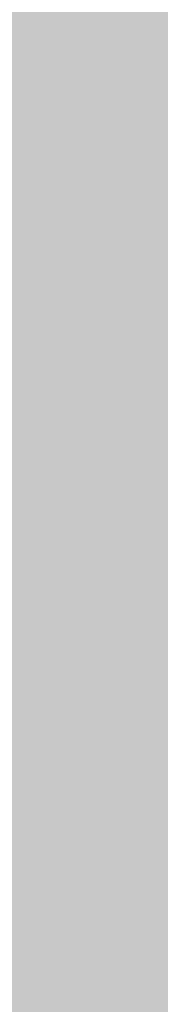
# Model space of a CAD drawing. Units: inches. Extents: x 2083 to 3317, y 1141 to 2115.
# Tile 168 of 256: x 3126.958245 to 3126.959398, y 1263.265937 to 1263.274018. Entities that reach past the tile are written whole.
import ezdxf

# ---------------------------------------------------------------- set-up
doc = ezdxf.new("R2010")
doc.units = ezdxf.units.IN
doc.layers.add('A-ANNO-DIMS', color=2, linetype='Continuous', lineweight=18)
doc.layers.add('A-WALL-PATT', color=251, linetype='Continuous', lineweight=13, true_color=0x636466)
doc.styles.get("Standard").update_dxf_attribs({"font": 'arial.ttf'})
doc.dimstyles.new('ISO-25', dxfattribs={"dimtxt": 12, "dimasz": 12, "dimexe": 1.25, "dimexo": 0.625, "dimtad": 1, "dimlunit": 3, "dimtxsty": 'Standard', "dimcen": 2.5, "dimadec": 0, "dimazin": 0, "dimtfac": 1, "dimtmove": 0, "dimatfit": 3, "dimfxl": 1, "dimarcsym": 0})

# ---------------------------------------------------------------- blocks, each defined once
blk = doc.blocks.new('*D26')
at = {"layer": 'A-ANNO-DIMS', "color": 0, "lineweight": -2, "transparency": 16777216}
for p, q in [((3088.985844, 1274.915092), (3088.985844, 1270.9519631)), ((3111.2400366, 1274.915092), (3111.2400366, 1270.9519631)), ((3076.985844, 1272.2019631), (2840.262447, 1272.2019631)), ((3111.2400366, 1272.2019631), (3088.985844, 1272.2019631)), ((3123.2400366, 1272.2019631), (3135.2400366, 1272.2019631))]:
    blk.add_line(p, q, dxfattribs=at)
at = {"layer": 'A-ANNO-DIMS', "color": 0, "transparency": 16777216}
for points in [[(3076.985844, 1274.2019631), (3076.985844, 1270.2019631), (3088.985844, 1272.2019631)], [(3123.2400366, 1274.2019631), (3123.2400366, 1270.2019631), (3111.2400366, 1272.2019631)]]:
    blk.add_solid(points, dxfattribs=at)
at = {"layer": 'Defpoints', "color": 0, "transparency": 16777216}
for p in [(3088.985844, 1275.540092), (3111.2400366, 1275.540092), (3088.985844, 1272.2019631)]:
    blk.add_point(p, dxfattribs=at)
at = {"layer": 'A-ANNO-DIMS', "color": 0, "transparency": 16777216, "insert": (2952.6241455, 1279.0316016), "char_height": 12, "attachment_point": 5}
blk.add_mtext('NIGHTSTAND 1\'-10 1/2" TYP.', dxfattribs=at)

msp = doc.modelspace()

# ---------------------------------------------------------------- hatches: boundary and pattern name
at = {"layer": 'A-WALL-PATT'}
h = msp.add_hatch(color=256, dxfattribs=at)
h.dxf.hatch_style = 1
h.paths.add_polyline_path([(3126.9597832, 2020.7613601), (2748.9597832, 2020.7613601), (2604.9597832, 2020.7613601), (2226.9597832, 2020.7613601), (2226.9597832, 1702.7613601), (2466.9597832, 1702.7613601), (2466.9597832, 1582.7613601), (2418.9597832, 1582.7613601), (2418.9597832, 1477.7613601), (2226.9597832, 1477.7613601), (2226.9597832, 1263.2613601), (2544.9597832, 1263.2613601), (2544.9597832, 1411.7613601), (2604.9597832, 1411.7613601), (2685.9597832, 1411.7613601), (2685.9597832, 1420.7613601), (2604.9597832, 1420.7613601), (2604.9597832, 1573.7613601), (2604.9597832, 1702.7613601), (2604.9597832, 2011.7613601), (2748.9597832, 2011.7613601), (2748.9597832, 1702.7613601), (2862.9597832, 1702.7613601), (2862.9597832, 1621.7613601), (2871.9597832, 1621.7613601), (2871.9597832, 1702.7613601), (2883.9597832, 1702.7613601), (2883.9597832, 1706.9394595, -0.026459), (2883.9597832, 1711.7613601), (2757.9597832, 1711.7613601), (2757.9597832, 1807.7613601), (2787.9597832, 1807.7613601), (2787.9597832, 1812.2613601), (2757.9597832, 1812.2613601), (2757.9597832, 2011.7613601), (2877.9597832, 2011.7613601), (2877.9597832, 1812.2613601), (2847.9597832, 1812.2613601), (2847.9597832, 1807.7613601), (2889.8357425, 1807.7613601), (2889.8357425, 1812.2613601), (2882.4597832, 1812.2613601), (2882.4597832, 2011.7613601), (3117.9597832, 2011.7613601), (3117.9597832, 1812.2613601), (2937.8357425, 1812.2613601), (2937.8357425, 1807.7613601), (2995.7097832, 1807.7613601), (2995.7097832, 1796.1176655), (3000.2097832, 1796.1176655), (3000.2097832, 1807.7613601), (3117.9597832, 1807.7613601), (3117.9597832, 1711.7613601), (3000.2097832, 1711.7613601), (3000.2097832, 1760.1176655), (2998.5727047, 1760.1176655, -0.020711), (2995.7097832, 1760.1176655), (2995.7097832, 1711.7613601), (2931.9597832, 1711.7613601), (2931.9597832, 1702.7613601), (3126.9597832, 1702.7613601)])
h.paths.add_polyline_path([(2471.4597832, 2011.7613601), (2471.4597832, 1810.0113601), (2462.7169357, 1810.0113601), (2462.7169357, 1805.5113601), (2505.9597832, 1805.5113601), (2505.9597832, 1810.0113601), (2475.9597832, 1810.0113601), (2475.9597832, 2011.7613601), (2595.9597832, 2011.7613601), (2595.9597832, 1810.0113601), (2565.9597832, 1810.0113601), (2565.9597832, 1805.5113601), (2595.9597832, 1805.5113601), (2595.9597832, 1711.7613601), (2235.9597832, 1711.7613601), (2235.9597832, 1805.5113601), (2353.7097832, 1805.5113601), (2353.7097832, 1796.0541624), (2358.2097832, 1796.0541624), (2358.2097832, 1805.5113601), (2414.7169357, 1805.5113601), (2414.7169357, 1810.0113601), (2235.9597832, 1810.0113601), (2235.9597832, 2011.7613601)], flags=16)
h.paths.add_polyline_path([(2270.2047343, 1994.6100082), (2270.2047343, 1970.6100082), (2246.2047343, 1970.6100082), (2246.2047343, 1994.6100082)], flags=0)
edge = h.paths.add_edge_path(flags=0)
edge.add_ellipse((2332.027391, 1899.7981761), major_axis=(-3.0429938, 3.0429938), ratio=0.16825245, start_angle=-161.3321656, end_angle=-156.3071136, ccw=False)
edge.add_ellipse((2333.0820373, 1898.7435297), major_axis=(-1.0546463, 1.0546463), ratio=0.453532097, start_angle=-123.371019, end_angle=-94.1591066)
edge = h.paths.add_edge_path(flags=0)
edge.add_ellipse((2332.027391, 1968.8762897), major_axis=(3.0429938, 3.0429938), ratio=0.16825245, start_angle=18.6678344, end_angle=23.6928864)
edge.add_spline(control_points=[(2332.9255964, 1970.6911045), (2332.2267681, 1970.3360997), (2330.8937087, 1969.6589054), (2328.4130803, 1970.9321376), (2327.2039345, 1967.7487119), (2324.7095965, 1969.9555886), (2322.5328223, 1967.012354), (2320.0128462, 1971.2958124), (2317.6803077, 1968.1578449), (2316.0405263, 1967.1020468), (2315.4269045, 1966.8096022)], knot_values=[0, 0, 0, 0, 2.267059, 4.324559, 6.685584, 8.878641, 11.121502, 14.300359, 17.755284, 19.732645, 19.732645, 19.732645, 19.732645], degree=3, periodic=0)
edge.add_ellipse((2332.027391, 1968.8762897), major_axis=(3.0429938, 3.0429938), ratio=0.16825245, start_angle=18.6678344, end_angle=23.6928864, ccw=False)
edge.add_ellipse((2333.0820373, 1969.930936), major_axis=(1.0546463, 1.0546463), ratio=0.453532097, start_angle=56.628981, end_angle=85.8408934, ccw=False)
edge = h.paths.add_edge_path(flags=0)
edge.add_spline(control_points=[(2296.4282874, 1967.9879081), (2293.6278045, 1965.3363137), (2287.7036238, 1959.727094), (2299.7438601, 1949.9956993), (2294.5325909, 1935.6685275), (2290.5732281, 1920.6035119), (2293.3941244, 1909.9736911), (2296.1854073, 1904.9665431)], knot_values=[0.099185, 0.099185, 0.099185, 0.099185, 0.345301, 0.619822, 0.982653, 1.386093, 1.810555, 1.810555, 1.810555, 1.810555], degree=3, periodic=0)
edge.add_spline(control_points=[(2296.1854073, 1904.9665431), (2297.3835817, 1902.6193002), (2298.0009694, 1901.9493116), (2298.5529698, 1901.4681549)], knot_values=[0.006246, 0.006246, 0.006246, 0.006246, 0.055476, 0.055476, 0.055476, 0.055476], degree=3, periodic=0)
edge.add_spline(control_points=[(2298.5529698, 1901.4681549), (2297.2586121, 1900.9232238), (2295.2252939, 1900.2321257), (2293.0602287, 1900.6142053), (2292.1014227, 1900.788415), (2292.0895776, 1900.790568)], knot_values=[0.312835, 0.312835, 0.312835, 0.312835, 0.40178, 0.474987, 0.475903, 0.475903, 0.475903, 0.475903], degree=3, periodic=0)
edge.add_arc((2292.7936464, 1904.6641088), 3.9370079, 215.4208969, 259.6981795, ccw=False)
edge.add_spline(control_points=[(2289.5853139, 1902.3823039), (2289.4766524, 1902.5350874), (2289.3684805, 1902.6880353), (2289.2608648, 1902.8411699)], knot_values=[0.102872, 0.102872, 0.102872, 0.102872, 0.116896, 0.116896, 0.116896, 0.116896], degree=3, periodic=0)
edge.add_spline(control_points=[(2289.2608648, 1902.8411699), (2288.6866042, 1902.5501922), (2287.6400477, 1902.0199025), (2285.8813368, 1901.8739536), (2283.8529717, 1901.5043521), (2281.7199871, 1899.7105375), (2278.4669913, 1899.492942), (2276.1571361, 1901.8832022), (2272.2589526, 1899.8040711), (2267.7776054, 1901.8431828), (2262.2438819, 1900.1840326), (2257.414927, 1901.7820606), (2254.318374, 1900.7261196), (2253.1782849, 1900.3373431)], knot_values=[0, 0, 0, 0, 1.907977, 3.477176, 5.261074, 7.972851, 11.680248, 13.717921, 16.939592, 22.789562, 27.502503, 33.595215, 37.145618, 37.145618, 37.145618, 37.145618], degree=3, periodic=0)
edge.add_line((2253.1782849, 1900.3373431), (2250.2442397, 1902.8411699))
edge.add_line((2250.2442397, 1902.8411699), (2250.2442397, 1965.8332959))
edge.add_line((2250.2442397, 1965.8332959), (2253.1782849, 1968.3371226))
edge.add_spline(control_points=[(2253.1782849, 1968.3371226), (2254.318374, 1967.9483462), (2257.414927, 1966.8924051), (2262.2438819, 1968.4904332), (2267.7776054, 1966.8312829), (2271.5267301, 1968.5372172), (2273.8759143, 1967.8282895), (2274.2067012, 1967.7276424)], knot_values=[0, 0, 0, 0, 0.09018, 0.244935, 0.364644, 0.513233, 0.537855, 0.537855, 0.537855, 0.537855], degree=3, periodic=0)
edge.add_arc((2274.3528869, 1963.7933495), 3.9370079, 72.0511336, 92.1279492, ccw=False)
edge.add_arc((2281.2969331, 1985.2300027), 18.5962982, 252.05113361, 288.56572166)
edge.add_arc((2292.3167172, 1956.0288805), 12.6460805, 71.02678788, 113.77821843, ccw=False)
edge = h.paths.add_edge_path(flags=0)
edge.add_spline(control_points=[(2274.8994147, 1951.8561946), (2275.066156, 1951.6165924), (2275.2326866, 1951.3765878), (2275.3979871, 1951.1358545)], knot_values=[1.409916, 1.409916, 1.409916, 1.409916, 1.43159, 1.43159, 1.43159, 1.43159], degree=3, periodic=0)
edge.add_spline(control_points=[(2275.3979871, 1951.1358545), (2275.7921055, 1950.5618854), (2276.1792311, 1949.9837745), (2276.5455462, 1949.3971029)], knot_values=[1.358238, 1.358238, 1.358238, 1.358238, 1.409916, 1.409916, 1.409916, 1.409916], degree=3, periodic=0)
edge.add_line((2276.5455462, 1949.3971029), (2277.437289, 1947.8621847))
edge.add_spline(control_points=[(2277.437289, 1947.8621847), (2276.3038341, 1945.6731147), (2274.6396979, 1942.4268817), (2274.631615, 1938.0938998), (2272.7991237, 1930.8515498), (2274.3564261, 1943.8970461), (2275.9476814, 1947.9233558), (2276.5455462, 1949.3971029)], knot_values=[0.005632, 0.005632, 0.005632, 0.005632, 0.186014, 0.266002, 0.357087, 0.59639, 0.739732, 0.739732, 0.739732, 0.739732], degree=3, periodic=0)
edge.add_spline(control_points=[(2276.5455462, 1949.3971029), (2276.1792311, 1949.9837745), (2275.7921055, 1950.5618854), (2275.3979871, 1951.1358545)], knot_values=[1.358238, 1.358238, 1.358238, 1.358238, 1.409916, 1.409916, 1.409916, 1.409916], degree=3, periodic=0)
edge.add_spline(control_points=[(2275.3979871, 1951.1358545), (2274.9425002, 1950.0804523), (2274.2077604, 1948.0252718), (2273.9346018, 1944.8514774), (2272.4685341, 1937.6274891), (2273.4662155, 1945.6964663), (2274.7006154, 1951.0594725), (2274.8994147, 1951.8561946)], knot_values=[0.104364, 0.104364, 0.104364, 0.104364, 0.189636, 0.269624, 0.36071, 0.600013, 0.644622, 0.644622, 0.644622, 0.644622], degree=3, periodic=0)
h.paths.add_polyline_path([(2269.1675139, 1963.1275729, -0.357527), (2268.170633, 1960.9763695, -0.092561), (2268.170633, 1939.4363249, -0.357527), (2269.1675139, 1937.2851215, -0.357527), (2267.0163105, 1938.2820024, -0.164785), (2254.6855813, 1938.2820024, -0.357527), (2252.5343779, 1937.2851215, -0.357527), (2253.5312587, 1939.4363249, -0.092561), (2253.5312587, 1960.9763695, -0.357527), (2252.5343779, 1963.1275729, -0.357527), (2254.6855813, 1962.130692, -0.164785), (2267.0163105, 1962.130692, -0.357527)], flags=0)
h.paths.add_polyline_path([(2248.8740679, 1967.8017998), (2248.8740679, 1957.0277095), (2249.4577833, 1957.0277095), (2249.4577833, 1911.6467562), (2248.8740679, 1911.6467562), (2248.8740679, 1900.8726659), (2246.5118632, 1900.8726659, 0.197327), (2244.1496584, 1902.4568734), (2244.1496584, 1966.2175923, 0.197327), (2246.5118632, 1967.8017998)], flags=0)
h.paths.add_polyline_path([(2269.1675139, 1931.3893442, -0.357527), (2268.170633, 1929.2381408, -0.092561), (2268.170633, 1907.6980962, -0.357527), (2269.1675139, 1905.5468928, -0.357527), (2267.0163105, 1906.5437737, -0.164785), (2254.6855813, 1906.5437737, -0.357527), (2252.5343779, 1905.5468928, -0.357527), (2253.5312587, 1907.6980962, -0.092561), (2253.5312587, 1929.2381408, -0.357527), (2252.5343779, 1931.3893442, -0.357527), (2254.6855813, 1930.3924634, -0.164785), (2267.0163105, 1930.3924634, -0.357527)], flags=0)
edge = h.paths.add_edge_path(flags=0)
edge.add_spline(control_points=[(2276.1968578, 1906.7237016), (2276.1681442, 1909.0289278), (2276.1140492, 1913.371852), (2270.5984171, 1924.9249783), (2273.9051746, 1919.0127787), (2275.9217115, 1916.2620626), (2275.4745699, 1912.4021495), (2277.2578735, 1910.3806206), (2276.6960436, 1908.2250358), (2276.6462176, 1906.8130226), (2276.6178249, 1906.0084068)], knot_values=[0, 0, 0, 0, 8.61026, 16.221274, 18.843057, 23.804898, 27.440828, 29.356102, 31.203478, 33.650687, 33.650687, 33.650687, 33.650687], degree=3, periodic=0)
edge.add_spline(control_points=[(2276.6178249, 1906.0084068), (2276.6233131, 1905.6241436), (2276.4977381, 1904.6286608), (2275.4417789, 1903.8547251), (2274.9373144, 1903.0804497), (2274.8590804, 1902.8411699)], knot_values=[0.156488, 0.156488, 0.156488, 0.156488, 0.184398, 0.231376, 0.250598, 0.250598, 0.250598, 0.250598], degree=3, periodic=0)
edge.add_line((2274.8590804, 1902.8411699), (2276.50598, 1902.8411699))
edge.add_spline(control_points=[(2276.50598, 1902.8411699), (2276.7883084, 1903.0849395), (2277.6650711, 1904.1251958), (2278.2495378, 1904.340738), (2277.6538719, 1908.5273866), (2278.15567, 1906.2278078), (2278.100464, 1905.2859484), (2278.8466748, 1904.0690054), (2277.8567853, 1903.4149482), (2277.8741909, 1902.9910497), (2277.9035616, 1902.8411699)], knot_values=[0.059574, 0.059574, 0.059574, 0.059574, 0.080753, 0.103741, 0.16972, 0.176036, 0.207137, 0.240474, 0.262341, 0.27366, 0.27366, 0.27366, 0.27366], degree=3, periodic=0)
edge.add_line((2277.9035616, 1902.8411699), (2280.0298255, 1902.8411699))
edge.add_spline(control_points=[(2280.0298255, 1902.8411699), (2279.8882214, 1903.088398), (2279.4992571, 1903.9815512), (2280.1522839, 1905.9393491), (2278.103615, 1909.6577572), (2279.7623946, 1907.185285), (2280.3279002, 1904.8748608), (2280.4851086, 1903.4895904), (2281.4632687, 1903.2494323), (2281.7583431, 1902.9364967), (2281.8340361, 1902.8411699)], knot_values=[0.013856, 0.013856, 0.013856, 0.013856, 0.034874, 0.088867, 0.107879, 0.126738, 0.158714, 0.193757, 0.217487, 0.226722, 0.226722, 0.226722, 0.226722], degree=3, periodic=0)
edge.add_spline(control_points=[(2281.8340361, 1902.8411699), (2281.7875348, 1902.8267029), (2281.6470224, 1902.7829881), (2281.3955272, 1902.85949), (2281.088077, 1902.9852418), (2280.7206826, 1903.060902), (2280.3334513, 1903.0257257), (2280.1247668, 1902.898879), (2280.0298255, 1902.8411699)], knot_values=[0, 0, 0, 0, 0.14413, 0.435517, 0.749276, 1.153046, 1.548371, 1.878348, 1.878348, 1.878348, 1.878348], degree=3, periodic=0)
edge.add_line((2280.0298255, 1902.8411699), (2277.9035616, 1902.8411699))
edge.add_spline(control_points=[(2277.9035616, 1902.8411699), (2277.892855, 1902.7958553), (2277.865396, 1902.6796374), (2277.6074793, 1902.6874828), (2277.2740503, 1902.8006999), (2276.8379209, 1902.6197745), (2276.5838074, 1902.7892611), (2276.50598, 1902.8411699)], knot_values=[0, 0, 0, 0, 0.127189, 0.326199, 0.628009, 1.24357, 1.515331, 1.515331, 1.515331, 1.515331], degree=3, periodic=0)
edge.add_line((2276.50598, 1902.8411699), (2274.8590804, 1902.8411699))
edge.add_spline(control_points=[(2274.8590804, 1902.8411699), (2274.8144367, 1902.8985868), (2274.7251297, 1903.013446), (2274.4934765, 1903.1189684), (2274.2442854, 1902.9605386), (2273.9371207, 1903.1849416), (2273.6140395, 1902.9831428), (2273.4083164, 1902.8830449), (2273.322254, 1902.8411699)], knot_values=[0, 0, 0, 0, 0.21843, 0.436957, 0.687977, 0.990379, 1.398396, 1.69185, 1.69185, 1.69185, 1.69185], degree=3, periodic=0)
edge.add_spline(control_points=[(2273.322254, 1902.8411699), (2273.6167403, 1903.445692), (2274.2739977, 1904.5382529), (2276.0272387, 1904.5737017), (2276.2069634, 1906.5836372), (2276.1968578, 1906.7237016)], knot_values=[0.012227, 0.012227, 0.012227, 0.012227, 0.059472, 0.106218, 0.134458, 0.134458, 0.134458, 0.134458], degree=3, periodic=0)
h.paths.add_polyline_path([(2270.7760538, 1897.7898284), (2270.7760538, 1873.7898284), (2246.7760538, 1873.7898284), (2246.7760538, 1897.7898284)], flags=0)
h.paths.add_polyline_path([(2353.7097832, 1760.0050593), (2353.7097832, 1760.0541624), (2358.2097832, 1760.0541624, -0.033729)], flags=0)
h.paths.add_polyline_path([(2321.8191188, 1737.5291862), (2341.9953271, 1737.5291862, -0.414214), (2343.2032727, 1736.3212406), (2343.2032727, 1721.0205964, -0.414214), (2341.9953271, 1719.8126508), (2321.8191188, 1719.8126508, -0.414214), (2320.6111732, 1721.0205964), (2320.6111732, 1736.3212406, -0.414214)], flags=0)
h.paths.add_polyline_path([(2324.2350099, 1736.3212406), (2339.5794359, 1736.3212406, -0.414214), (2341.9953271, 1733.9053494), (2341.9953271, 1725.4497302, -0.414214), (2339.5794359, 1723.033839), (2333.6805885, 1723.033839), (2333.8453172, 1722.0454666, -0.870646), (2335.4253988, 1721.8258934, -0.767327), (2333.922694, 1721.4232449), (2331.2910241, 1721.4232449, -0.767327), (2329.7883193, 1721.8258934, -0.870646), (2331.3684009, 1722.0454666), (2331.5331296, 1723.033839), (2324.2350099, 1723.033839, -0.414214), (2321.8191188, 1725.4497302), (2321.8191188, 1733.9053494, -0.414214)], flags=0)
h.paths.add_polyline_path([(2570.4837892, 1928.6154443), (2589.6837892, 1928.6154443), (2590.1688286, 1928.6154443), (2590.1688286, 1904.9933971), (2570.4837892, 1904.9933971)], flags=0)
h.paths.add_polyline_path([(2574.4473242, 1927.2638215, -1), (2572.8288357, 1927.2638215, -1)], flags=0)
h.paths.add_polyline_path([(2573.0898665, 1926.9408768), (2573.925032, 1927.7760423), (2574.1477428, 1927.5533315), (2573.3125773, 1926.718166)], flags=0)
h.paths.add_polyline_path([(2578.7790648, 1919.7296175, -1), (2571.5916632, 1919.7296175, -1)], flags=0)
h.paths.add_polyline_path([(2578.385364, 1919.7296175, -1), (2571.985364, 1919.7296175, -1)], flags=0)
h.paths.add_polyline_path([(2331.5957638, 1729.4762156, -1), (2333.6179542, 1729.4762156, -1)], flags=0)
h.paths.add_polyline_path([(2578.0342282, 1927.2638215, -1), (2576.4157396, 1927.2638215, -1)], flags=0)
h.paths.add_polyline_path([(2576.6888513, 1927.5310886), (2576.9115621, 1927.7537993), (2577.7467276, 1926.9186339), (2577.5240168, 1926.6959231)], flags=0)
h.paths.add_polyline_path([(2578.1390648, 1909.8595388, -1), (2572.2316632, 1909.8595388, -1)], flags=0)
h.paths.add_polyline_path([(2577.745364, 1909.8595388, -1), (2572.625364, 1909.8595388, -1)], flags=0)
h.paths.add_polyline_path([(2583.7977179, 1927.2638215, -1), (2582.1792294, 1927.2638215, -1)], flags=0)
h.paths.add_polyline_path([(2582.7186487, 1927.7537993), (2583.5538142, 1926.9186339), (2583.3311034, 1926.6959231), (2582.4959379, 1927.5310886)], flags=0)
h.paths.add_polyline_path([(2582.4959379, 1927.5310886), (2582.7186487, 1927.7537993), (2583.5538142, 1926.9186339), (2583.3311034, 1926.6959231)], flags=0)
h.paths.add_polyline_path([(2587.7390648, 1920.5296175, -1), (2581.8316632, 1920.5296175, -1)], flags=0)
h.paths.add_polyline_path([(2587.345364, 1920.5296175, -1), (2582.225364, 1920.5296175, -1)], flags=0)
h.paths.add_polyline_path([(2587.3846219, 1927.2638215, -1), (2585.7661333, 1927.2638215, -1)], flags=0)
h.paths.add_polyline_path([(2586.0819925, 1926.9802469), (2586.917158, 1927.8154124), (2587.1398688, 1927.5927016), (2586.3047033, 1926.7575361)], flags=0)
h.paths.add_polyline_path([(2588.3790648, 1910.6595388, -1), (2581.1916632, 1910.6595388, -1)], flags=0)
h.paths.add_polyline_path([(2587.985364, 1910.6595388, -1), (2581.585364, 1910.6595388, -1)], flags=0)
h.paths.add_polyline_path([(2417.1677288, 1729.4778955), (2437.3439372, 1729.4778955, -0.414214), (2438.5518828, 1728.2699499), (2438.5518828, 1712.9693057, -0.414214), (2437.3439372, 1711.7613601), (2417.1677288, 1711.7613601, -0.414214), (2415.9597832, 1712.9693057), (2415.9597832, 1728.2699499, -0.414214)], flags=0)
h.paths.add_polyline_path([(2419.58362, 1728.2699499), (2434.928046, 1728.2699499, -0.414214), (2437.3439372, 1725.8540587), (2437.3439372, 1717.3984395, -0.414214), (2434.928046, 1714.9825483), (2429.0291985, 1714.9825483), (2429.1939273, 1713.9941758, -0.870646), (2430.7740089, 1713.7746027, -0.767327), (2429.2713041, 1713.3719542), (2426.6396342, 1713.3719542, -0.767327), (2425.1369294, 1713.7746027, -0.870646), (2426.717011, 1713.9941758), (2426.8817397, 1714.9825483), (2419.58362, 1714.9825483, -0.414214), (2417.1677288, 1717.3984395), (2417.1677288, 1725.8540587, -0.414214)], flags=0)
h.paths.add_polyline_path([(2419.58362, 1728.2699499), (2434.928046, 1728.2699499, -0.414214), (2437.3439372, 1725.8540587), (2437.3439372, 1717.3984395, -0.414214), (2434.928046, 1714.9825483), (2429.0291985, 1714.9825483), (2428.3581177, 1719.0090337), (2427.5528206, 1719.0090337), (2426.8817397, 1714.9825483), (2419.58362, 1714.9825483, -0.414214), (2417.1677288, 1717.3984395), (2417.1677288, 1725.8540587, -0.414214)], flags=0)
h.paths.add_polyline_path([(2426.9443739, 1721.4249248, -1), (2428.9665643, 1721.4249248, -1)], flags=0)
h.paths.add_polyline_path([(2475.9597832, 1702.7613601), (2595.9597832, 1702.7613601), (2595.9597832, 1582.7613601), (2475.9597832, 1582.7613601)], flags=16)
h.paths.add_polyline_path([(2427.9597832, 1573.7613601), (2595.9597832, 1573.7613601), (2595.9597832, 1468.7613601), (2595.9597832, 1420.7613601), (2384.4597832, 1420.7613601), (2384.4597832, 1468.7613601), (2427.9597832, 1468.7613601)], flags=16)
h.paths.add_polyline_path([(2379.9597832, 1468.7613601), (2379.9597832, 1420.7613601), (2235.9597832, 1420.7613601), (2235.9597832, 1468.7613601)], flags=16)
h.paths.add_polyline_path([(2317.8159962, 1466.695767), (2337.9922045, 1466.695767, -0.414214), (2339.2001501, 1465.4878214), (2339.2001501, 1450.1871771, -0.414214), (2337.9922045, 1448.9792315), (2317.8159962, 1448.9792315, -0.414214), (2316.6080506, 1450.1871771), (2316.6080506, 1465.4878214, -0.414214)], flags=0)
h.paths.add_polyline_path([(2320.2318874, 1465.4878214), (2335.5763133, 1465.4878214, -0.414214), (2337.9922045, 1463.0719302), (2337.9922045, 1454.616311, -0.414214), (2335.5763133, 1452.2004198), (2329.6774659, 1452.2004198), (2329.8421946, 1451.2120473, -0.870646), (2331.4222762, 1450.9924742, -0.767327), (2329.9195714, 1450.5898257), (2327.2879015, 1450.5898257, -0.767327), (2325.7851967, 1450.9924742, -0.870646), (2327.3652783, 1451.2120473), (2327.530007, 1452.2004198), (2320.2318874, 1452.2004198, -0.414214), (2317.8159962, 1454.616311), (2317.8159962, 1463.0719302, -0.414214)], flags=0)
h.paths.add_polyline_path([(2320.2318874, 1465.4878214), (2335.5763133, 1465.4878214, -0.414214), (2337.9922045, 1463.0719302), (2337.9922045, 1454.616311, -0.414214), (2335.5763133, 1452.2004198), (2329.6774659, 1452.2004198), (2329.006385, 1456.2269051), (2328.2010879, 1456.2269051), (2327.530007, 1452.2004198), (2320.2318874, 1452.2004198, -0.414214), (2317.8159962, 1454.616311), (2317.8159962, 1463.0719302, -0.414214)], flags=0)
h.paths.add_polyline_path([(2327.5926413, 1458.6427963, -1), (2329.6148317, 1458.6427963, -1)], flags=0)
h.paths.add_polyline_path([(2244.4117436, 1433.3404531), (2241.9209449, 1433.3404531, -0.414214), (2240.0178562, 1435.2435418), (2240.0178562, 1440.9528078, -0.414211), (2241.920925, 1442.8558965), (2244.4117436, 1442.8558965, -1.976472)], flags=0)
h.paths.add_polyline_path([(2245.3568884, 1434.3975358, -0.414214), (2245.3568884, 1441.7988138, -2.144098)], flags=0)
h.paths.add_polyline_path([(2535.9597832, 1416.2613601), (2535.9597832, 1272.2613601), (2235.9597832, 1272.2613601), (2235.9597832, 1416.2613601)], flags=16)
h.paths.add_polyline_path([(2260.1195614, 1384.2928413), (2260.1195614, 1362.0386487), (2237.8653688, 1362.0386487), (2237.8653688, 1384.2928413)], flags=0)
edge = h.paths.add_edge_path(flags=0)
edge.add_line((2318.2518466, 1362.0932983), (2318.1457968, 1362.0009726))
edge.add_ellipse((2317.4451158, 1360.4310442), major_axis=(2.8216404, 2.8216404), ratio=0.16825245, start_angle=18.6678344, end_angle=20.9481273, ccw=False)
edge.add_ellipse((2318.4230451, 1361.4089735), major_axis=(0.9779293, 0.9779293), ratio=0.453532097, start_angle=56.628981, end_angle=70.2262012, ccw=False)
edge = h.paths.add_edge_path(flags=0)
edge.add_line((2319.1073699, 1295.5710784), (2319.0150442, 1295.6771282))
edge.add_ellipse((2317.4451158, 1296.3778091), major_axis=(-2.8216404, 2.8216404), ratio=0.16825245, start_angle=-161.3321656, end_angle=-159.0518727, ccw=False)
edge.add_ellipse((2318.4230451, 1295.3998798), major_axis=(-0.9779293, 0.9779293), ratio=0.453532097, start_angle=-123.371019, end_angle=-109.7737988)
edge = h.paths.add_edge_path(flags=0)
edge.add_spline(control_points=[(2284.2103489, 1301.1702189), (2284.5806878, 1300.444719), (2284.8911891, 1299.8920243), (2285.159553, 1299.4610182)], knot_values=[0.039066, 0.039066, 0.039066, 0.039066, 0.055476, 0.055476, 0.055476, 0.055476], degree=3, periodic=0)
edge.add_line((2285.159553, 1299.4610182), (2284.2103489, 1301.1702189))
edge = h.paths.add_edge_path(flags=0)
edge.add_line((2280.4124579, 1297.2980125), (2283.3699905, 1297.0361216))
edge.add_line((2283.3699905, 1297.0361216), (2286.4056902, 1297.9263104))
edge.add_spline(control_points=[(2286.4056902, 1297.9263104), (2285.305487, 1297.4631193), (2284.3447774, 1297.1291508), (2283.3699905, 1297.0361216)], knot_values=[0.394369, 0.394369, 0.394369, 0.394369, 0.475903, 0.475903, 0.475903, 0.475903], degree=3, periodic=0)
edge.add_spline(control_points=[(2283.3699905, 1297.0361216), (2283.2813895, 1297.027666), (2282.316289, 1296.9573356), (2281.3125019, 1297.1344787), (2280.4234414, 1297.2960161), (2280.4124579, 1297.2980125)], knot_values=[0.312835, 0.312835, 0.312835, 0.312835, 0.320246, 0.393453, 0.394369, 0.394369, 0.394369, 0.394369], degree=3, periodic=0)
edge = h.paths.add_edge_path(flags=0)
edge.add_line((2284.4355615, 1359.6072854), (2280.4462909, 1355.328047))
edge.add_line((2280.4462909, 1355.328047), (2279.5799868, 1351.0177544))
edge.add_line((2279.5799868, 1351.0177544), (2282.4129737, 1346.5804327))
edge.add_spline(control_points=[(2282.4129737, 1346.5804327), (2283.1533308, 1345.5892358), (2284.2528957, 1344.0288973), (2284.801037, 1342.3871671), (2284.9351625, 1341.8055443)], knot_values=[1.240098, 1.240098, 1.240098, 1.240098, 1.332892, 1.382712, 1.382712, 1.382712, 1.382712], degree=3, periodic=0)
edge.add_spline(control_points=[(2284.9351625, 1341.8055443), (2285.3191079, 1340.1406002), (2285.2330291, 1338.4092041), (2284.9099384, 1336.6541222)], knot_values=[1.097484, 1.097484, 1.097484, 1.097484, 1.240098, 1.240098, 1.240098, 1.240098], degree=3, periodic=0)
edge.add_spline(control_points=[(2284.9099384, 1336.6541222), (2284.5868478, 1334.8990403), (2284.0267453, 1333.1202725), (2283.4626437, 1331.3605849)], knot_values=[0.95487, 0.95487, 0.95487, 0.95487, 1.097484, 1.097484, 1.097484, 1.097484], degree=3, periodic=0)
edge.add_line((2283.4626437, 1331.3605849), (2281.8903759, 1326.153357))
edge.add_line((2281.8903759, 1326.153357), (2280.7562592, 1321.0560888))
edge.add_line((2280.7562592, 1321.0560888), (2280.2992048, 1316.0019772))
edge.add_line((2280.2992048, 1316.0019772), (2280.7159327, 1310.9500678))
edge.add_line((2280.7159327, 1310.9500678), (2282.0280939, 1305.9721367))
edge.add_line((2282.0280939, 1305.9721367), (2284.2103489, 1301.1702189))
edge.add_spline(control_points=[(2284.2103489, 1301.1702189), (2283.3407305, 1302.7301854), (2282.6119044, 1304.3364933), (2282.0280939, 1305.9721367)], knot_values=[0.099185, 0.099185, 0.099185, 0.099185, 0.241799, 0.241799, 0.241799, 0.241799], degree=3, periodic=0)
edge.add_spline(control_points=[(2282.0280939, 1305.9721367), (2281.4442835, 1307.6077801), (2281.0054886, 1309.2727591), (2280.7159327, 1310.9500678)], knot_values=[0.241799, 0.241799, 0.241799, 0.241799, 0.384413, 0.384413, 0.384413, 0.384413], degree=3, periodic=0)
edge.add_spline(control_points=[(2280.7159327, 1310.9500678), (2280.4332411, 1312.5876134), (2280.2893863, 1314.2769594), (2280.2988938, 1315.9620324), (2280.2992048, 1316.0019772)], knot_values=[0.384413, 0.384413, 0.384413, 0.384413, 0.523647, 0.527028, 0.527028, 0.527028, 0.527028], degree=3, periodic=0)
edge.add_spline(control_points=[(2280.2992048, 1316.0019772), (2280.3123257, 1317.6869552), (2280.4778706, 1319.3679256), (2280.7562592, 1321.0560888)], knot_values=[0.527028, 0.527028, 0.527028, 0.527028, 0.669642, 0.669642, 0.669642, 0.669642], degree=3, periodic=0)
edge.add_spline(control_points=[(2280.7562592, 1321.0560888), (2281.0346478, 1322.7442519), (2281.4258801, 1324.4396079), (2281.8903759, 1326.153357)], knot_values=[0.669642, 0.669642, 0.669642, 0.669642, 0.812256, 0.812256, 0.812256, 0.812256], degree=3, periodic=0)
edge.add_spline(control_points=[(2281.8903759, 1326.153357), (2282.2643834, 1327.5332507), (2282.7878702, 1329.2618097), (2283.352751, 1331.0177803), (2283.4626437, 1331.3605849)], knot_values=[0.812256, 0.812256, 0.812256, 0.812256, 0.927087, 0.95487, 0.95487, 0.95487, 0.95487], degree=3, periodic=0)
edge.add_line((2283.4626437, 1331.3605849), (2284.9099384, 1336.6541222))
edge.add_line((2284.9099384, 1336.6541222), (2284.9351625, 1341.8055443))
edge.add_line((2284.9351625, 1341.8055443), (2282.4129737, 1346.5804327))
edge.add_spline(control_points=[(2282.4129737, 1346.5804327), (2281.2751273, 1348.1037918), (2280.0784467, 1349.5703178), (2279.5799868, 1351.0177544)], knot_values=[1.382712, 1.382712, 1.382712, 1.382712, 1.525326, 1.525326, 1.525326, 1.525326], degree=3, periodic=0)
edge.add_spline(control_points=[(2279.5799868, 1351.0177544), (2279.4432818, 1351.4147209), (2279.1363124, 1352.856922), (2279.7351897, 1354.2903851), (2280.4462909, 1355.328047)], knot_values=[1.525326, 1.525326, 1.525326, 1.525326, 1.564439, 1.667941, 1.667941, 1.667941, 1.667941], degree=3, periodic=0)
edge.add_spline(control_points=[(2280.4462909, 1355.328047), (2281.4261132, 1356.7578354), (2282.9308373, 1358.1825604), (2284.4355615, 1359.6072854)], knot_values=[1.667941, 1.667941, 1.667941, 1.667941, 1.810555, 1.810555, 1.810555, 1.810555], degree=3, periodic=0)
edge.add_arc((2280.6230749, 1348.518181), 11.7261796, 71.02678788, 113.77821843)
edge.add_arc((2270.4048917, 1375.5951559), 17.2435667, 252.05113361, 288.56572166, ccw=False)
edge.add_arc((2263.9659692, 1355.7178471), 3.6506221, 72.0511336, 92.1279492)
edge.add_arc((2263.9659692, 1355.7178471), 3.6506221, 92.1279492, 177.98513)
edge.add_spline(control_points=[(2260.3176041, 1355.8461989), (2260.2604169, 1354.2206683), (2260.551278, 1350.1865469), (2262.9993445, 1346.7662507), (2264.4727415, 1344.6490245)], knot_values=[1.43159, 1.43159, 1.43159, 1.43159, 1.564144, 1.770695, 1.770695, 1.770695, 1.770695], degree=3, periodic=0)
edge.add_line((2264.4727415, 1344.6490245), (2264.9355904, 1343.9825301))
edge.add_spline(control_points=[(2263.8010444, 1340.2481052), (2263.8432379, 1340.5140884), (2264.0672444, 1341.7564652), (2264.5126928, 1343.0024532), (2264.9350468, 1343.9810834)], knot_values=[0.53657, 0.53657, 0.53657, 0.53657, 0.559349, 0.644622, 0.644622, 0.644622, 0.644622], degree=3, periodic=0)
edge.add_spline(control_points=[(2264.9350468, 1343.9810834), (2265.1177715, 1343.7149747), (2265.2988751, 1343.4479058), (2265.4767562, 1343.1793646)], knot_values=[1.384077, 1.384077, 1.384077, 1.384077, 1.409916, 1.409916, 1.409916, 1.409916], degree=3, periodic=0)
edge.add_spline(control_points=[(2265.4767562, 1343.1793646), (2265.6546373, 1342.9108234), (2265.8292958, 1342.64081), (2265.9991301, 1342.368812)], knot_values=[1.358238, 1.358238, 1.358238, 1.358238, 1.384077, 1.384077, 1.384077, 1.384077], degree=3, periodic=0)
edge.add_line((2265.9991301, 1342.368812), (2266.8260057, 1340.9455468))
edge.add_spline(control_points=[(2266.8260057, 1340.9455468), (2268.894401, 1337.0896912), (2271.3981727, 1325.8430009), (2270.5161644, 1310.5685568), (2275.9193759, 1301.860609), (2277.7895113, 1299.1994495)], knot_values=[0.116896, 0.116896, 0.116896, 0.116896, 0.472987, 1.050969, 1.313793, 1.313793, 1.313793, 1.313793], degree=3, periodic=0)
edge.add_spline(control_points=[(2277.7895113, 1299.1994495), (2277.8394051, 1299.1284519), (2277.8894277, 1299.0574975), (2277.9395717, 1298.9865839)], knot_values=[0.109884, 0.109884, 0.109884, 0.109884, 0.116896, 0.116896, 0.116896, 0.116896], degree=3, periodic=0)
edge.add_line((2277.9395717, 1298.9865839), (2277.7888489, 1299.1991139))
edge.add_spline(control_points=[(2277.7888489, 1299.1991139), (2277.2565819, 1298.9294144), (2276.2863504, 1298.4379024), (2275.0393517, 1298.3344186), (2274.3833299, 1298.2388951), (2274.2152543, 1298.209338)], knot_values=[33.12187, 33.12187, 33.12187, 33.12187, 35.029056, 36.598255, 37.144827, 37.144827, 37.144827, 37.144827], degree=3, periodic=0)
edge.add_line((2274.2152543, 1298.209338), (2273.073147, 1297.8929607))
edge.add_spline(control_points=[(2273.073147, 1297.8929607), (2272.3229363, 1297.579784), (2271.0391507, 1296.5105078), (2269.2483948, 1296.2260622), (2268.4231004, 1296.3746543)], knot_values=[26.532584, 26.532584, 26.532584, 26.532584, 29.198919, 31.839101, 31.839101, 31.839101, 31.839101], degree=3, periodic=0)
edge.add_line((2268.4231004, 1296.3746543), (2263.8785014, 1297.4575338))
edge.add_spline(control_points=[(2263.8785014, 1297.4575338), (2263.5560769, 1297.3594345), (2261.8603064, 1296.8386943), (2260.2387805, 1297.2824073), (2258.9334543, 1297.5164611)], knot_values=[15.919551, 15.919551, 15.919551, 15.919551, 16.939592, 21.226067, 21.226067, 21.226067, 21.226067], degree=3, periodic=0)
edge.add_line((2258.9334543, 1297.5164611), (2254.0552332, 1297.3290098))
edge.add_spline(control_points=[(2254.0552332, 1297.3290098), (2253.7555255, 1297.295815), (2252.1136834, 1297.1651738), (2250.4618687, 1297.5442209), (2249.1296862, 1297.6678818)], knot_values=[5.306517, 5.306517, 5.306517, 5.306517, 6.276435, 10.613034, 10.613034, 10.613034, 10.613034], degree=3, periodic=0)
edge.add_line((2249.1296862, 1297.6678818), (2244.3316495, 1296.8777561))
edge.add_line((2244.3316495, 1296.8777561), (2241.6110326, 1299.1994495))
edge.add_line((2241.6110326, 1299.1994495), (2241.6110326, 1357.6094038))
edge.add_line((2241.6110326, 1357.6094038), (2244.3316495, 1359.9310973))
edge.add_line((2244.3316495, 1359.9310973), (2252.7288228, 1359.5426917))
edge.add_spline(control_points=[(2252.7288228, 1359.5426917), (2252.8709387, 1359.5464396), (2253.3057402, 1359.5481716), (2253.7398447, 1359.5142744), (2254.0317419, 1359.4824261)], knot_values=[0.233291, 0.233291, 0.233291, 0.233291, 0.244935, 0.268927, 0.268927, 0.268927, 0.268927], degree=3, periodic=0)
edge.add_line((2254.0317419, 1359.4824261), (2259.5871899, 1359.4163899))
edge.add_spline(control_points=[(2259.5871899, 1359.4163899), (2260.6770676, 1359.6285026), (2262.0731971, 1359.8970025), (2263.5236925, 1359.4592776), (2263.8304173, 1359.3659518)], knot_values=[0.422516, 0.422516, 0.422516, 0.422516, 0.513233, 0.537855, 0.537855, 0.537855, 0.537855], degree=3, periodic=0)
edge.add_arc((2263.9659692, 1355.7178471), 3.6506221, 72.0511336, 92.1279492, ccw=False)
edge.add_arc((2270.4048917, 1375.5951559), 17.2435667, 252.05113361, 288.56572166)
edge.add_arc((2280.6230749, 1348.518181), 11.7261796, 71.02678788, 113.77821843, ccw=False)
h.paths.add_polyline_path([(2240.3405298, 1359.4347149), (2240.3405298, 1349.4443532), (2240.8817846, 1349.4443532), (2240.8817846, 1307.3645001), (2240.3405298, 1307.3645001), (2240.3405298, 1297.3741385), (2238.1501565, 1297.3741385, 0.197327), (2235.9597832, 1298.8431076), (2235.9597832, 1357.9657458, 0.197327), (2238.1501565, 1359.4347149)], flags=0)
h.paths.add_polyline_path([(2259.1577904, 1355.1005005, -0.357527), (2258.2334246, 1353.1057799, -0.092561), (2258.2334246, 1333.1326007, -0.357527), (2259.1577904, 1331.1378801, -0.357527), (2257.1630698, 1332.0622458, -0.164785), (2245.7293022, 1332.0622458, -0.357527), (2243.7345816, 1331.1378801, -0.357527), (2244.6589474, 1333.1326007, -0.092561), (2244.6589474, 1353.1057799, -0.357527), (2243.7345816, 1355.1005005, -0.357527), (2245.7293022, 1354.1761347, -0.164785), (2257.1630698, 1354.1761347, -0.357527)], flags=0)
edge = h.paths.add_edge_path(flags=0)
edge.add_line((2265.9991301, 1342.368812), (2266.8260057, 1340.9455468))
edge.add_line((2266.8260057, 1340.9455468), (2265.3075567, 1337.8140664))
edge.add_line((2265.3075567, 1337.8140664), (2264.358232, 1334.6529388))
edge.add_line((2264.358232, 1334.6529388), (2264.2620123, 1333.7997046))
edge.add_spline(control_points=[(2264.2620123, 1333.7997046), (2264.2083565, 1333.187055), (2264.1620602, 1332.3655252), (2264.0071444, 1331.4139326), (2263.9690487, 1331.2018338)], knot_values=[0.464444, 0.464444, 0.464444, 0.464444, 0.516691, 0.531608, 0.531608, 0.531608, 0.531608], degree=3, periodic=0)
edge.add_spline(control_points=[(2263.9690487, 1331.2018338), (2263.7745349, 1330.1188727), (2263.4243703, 1328.7908386), (2263.2574202, 1328.5306516), (2263.2340282, 1328.5146115)], knot_values=[0.372682, 0.372682, 0.372682, 0.372682, 0.44885, 0.464444, 0.464444, 0.464444, 0.464444], degree=3, periodic=0)
edge.add_spline(control_points=[(2263.2340282, 1328.5146115), (2263.096382, 1328.4202271), (2263.1311696, 1329.3014765), (2263.2749528, 1330.6157493)], knot_values=[0.280919, 0.280919, 0.280919, 0.280919, 0.372682, 0.372682, 0.372682, 0.372682], degree=3, periodic=0)
edge.add_spline(control_points=[(2263.2749528, 1330.6157493), (2263.4187361, 1331.930022), (2263.6715151, 1333.677318), (2263.9698519, 1335.3150268)], knot_values=[0.189157, 0.189157, 0.189157, 0.189157, 0.280919, 0.280919, 0.280919, 0.280919], degree=3, periodic=0)
edge.add_spline(control_points=[(2263.9698519, 1335.3150268), (2264.1004958, 1336.0321917), (2264.4187827, 1337.6219113), (2264.7548476, 1338.8644304), (2264.9474193, 1339.4911244)], knot_values=[0.097394, 0.097394, 0.097394, 0.097394, 0.137578, 0.189157, 0.189157, 0.189157, 0.189157], degree=3, periodic=0)
edge.add_spline(control_points=[(2264.9474193, 1339.4911244), (2265.2900171, 1340.6060546), (2265.6442376, 1341.4939958), (2265.9991301, 1342.368812)], knot_values=[0.005632, 0.005632, 0.005632, 0.005632, 0.097394, 0.097394, 0.097394, 0.097394], degree=3, periodic=0)
h.paths.add_polyline_path([(2259.1577904, 1325.6709733, -0.357527), (2258.2334246, 1323.6762527, -0.092561), (2258.2334246, 1303.7030735, -0.357527), (2259.1577904, 1301.7083529, -0.357527), (2257.1630698, 1302.6327186, -0.164785), (2245.7293022, 1302.6327186, -0.357527), (2243.7345816, 1301.7083529, -0.357527), (2244.6589474, 1303.7030735, -0.092561), (2244.6589474, 1323.6762527, -0.357527), (2243.7345816, 1325.6709733, -0.357527), (2245.7293022, 1324.7466075, -0.164785), (2257.1630698, 1324.7466075, -0.357527)], flags=0)
edge = h.paths.add_edge_path(flags=0)
edge.add_spline(control_points=[(2261.7089377, 1317.3114208), (2261.6794818, 1317.4175798), (2261.7618581, 1317.3885347), (2262.4907358, 1316.0898725), (2262.962185, 1315.3008975)], knot_values=[14.955861, 14.955861, 14.955861, 14.955861, 16.221274, 18.694826, 18.694826, 18.694826, 18.694826], degree=3, periodic=0)
edge.add_spline(control_points=[(2262.962185, 1315.3008975), (2262.9904374, 1315.2536169), (2263.7020958, 1314.0673762), (2264.3489834, 1313.1271533), (2264.7300545, 1312.1641544)], knot_values=[18.694826, 18.694826, 18.694826, 18.694826, 18.843057, 22.433791, 22.433791, 22.433791, 22.433791], degree=3, periodic=0)
edge.add_spline(control_points=[(2264.7300545, 1312.1641544), (2264.8755649, 1311.7964373), (2265.1768733, 1310.7698073), (2265.1430689, 1309.5592623), (2265.2477363, 1308.8241926)], knot_values=[22.433791, 22.433791, 22.433791, 22.433791, 23.804898, 26.172756, 26.172756, 26.172756, 26.172756], degree=3, periodic=0)
edge.add_line((2265.2477363, 1308.8241926), (2265.8507741, 1307.1718879))
edge.add_spline(control_points=[(2265.8507741, 1307.1718879), (2266.0650246, 1306.8216779), (2266.3843872, 1306.3322461), (2266.4244001, 1305.7805489), (2266.4203688, 1305.6112163)], knot_values=[28.062562, 28.062562, 28.062562, 28.062562, 29.356102, 29.911721, 29.911721, 29.911721, 29.911721], degree=3, periodic=0)
edge.add_spline(control_points=[(2266.4203688, 1305.6112163), (2266.4161162, 1305.4325896), (2266.393999, 1305.2499979), (2266.3647773, 1305.0658571)], knot_values=[29.911721, 29.911721, 29.911721, 29.911721, 30.497837, 30.497837, 30.497837, 30.497837], degree=3, periodic=0)
edge.add_line((2266.3647773, 1305.0658571), (2266.0661511, 1302.1362954))
edge.add_spline(control_points=[(2266.0661511, 1302.1362954), (2266.0712401, 1301.7799843), (2265.9980761, 1301.1999847), (2265.6632664, 1300.7589613), (2265.5089084, 1300.5858824)], knot_values=[0.156488, 0.156488, 0.156488, 0.156488, 0.184398, 0.203543, 0.203543, 0.203543, 0.203543], degree=3, periodic=0)
edge.add_line((2265.5089084, 1300.5858824), (2264.4353411, 1299.1994495))
edge.add_line((2264.4353411, 1299.1994495), (2265.962442, 1299.1994495))
edge.add_line((2265.962442, 1299.1994495), (2267.3359898, 1301.1752758))
edge.add_line((2267.3359898, 1301.1752758), (2267.3116668, 1301.9862366))
edge.add_spline(control_points=[(2267.3116668, 1301.9862366), (2267.261111, 1302.8623959), (2267.1602121, 1303.7371316), (2267.2714865, 1303.3258962)], knot_values=[0.126229, 0.126229, 0.126229, 0.126229, 0.166617, 0.166617, 0.166617, 0.166617], degree=3, periodic=0)
edge.add_spline(control_points=[(2267.2714865, 1303.3258962), (2267.2800347, 1303.2943047), (2267.3097851, 1303.1753659), (2267.3734504, 1302.8836084), (2267.4061233, 1302.6828291), (2267.4179259, 1302.6010251)], knot_values=[0.166617, 0.166617, 0.166617, 0.166617, 0.16972, 0.176036, 0.180765, 0.180765, 0.180765, 0.180765], degree=3, periodic=0)
edge.add_spline(control_points=[(2267.7438914, 1300.9875045), (2267.6875832, 1301.1509426), (2267.4805198, 1301.6566644), (2267.4837514, 1302.1447877), (2267.4179259, 1302.6010251)], knot_values=[0.180765, 0.180765, 0.180765, 0.180765, 0.193767, 0.220139, 0.220139, 0.220139, 0.220139], degree=3, periodic=0)
edge.add_line((2267.4179259, 1302.6010251), (2267.7438914, 1300.9875045))
edge.add_spline(control_points=[(2267.7438914, 1300.9875045), (2267.8319608, 1300.7318778), (2267.9320205, 1300.3099042), (2267.5548409, 1299.9745185), (2267.429366, 1299.8292073)], knot_values=[0.220139, 0.220139, 0.220139, 0.220139, 0.240474, 0.25489, 0.25489, 0.25489, 0.25489], degree=3, periodic=0)
edge.add_line((2267.429366, 1299.8292073), (2267.2583608, 1299.1994495))
edge.add_line((2267.2583608, 1299.1994495), (2269.229956, 1299.1994495))
edge.add_spline(control_points=[(2269.229956, 1299.1994495), (2269.0986525, 1299.4286938), (2268.842774, 1300.0162509), (2269.0115749, 1300.9159235), (2268.9467957, 1301.6607397)], knot_values=[0.013856, 0.013856, 0.013856, 0.013856, 0.034874, 0.067073, 0.067073, 0.067073, 0.067073], degree=3, periodic=0)
edge.add_line((2268.9467957, 1301.6607397), (2268.4315815, 1303.6031089))
edge.add_spline(control_points=[(2268.4315815, 1303.6031089), (2268.1755957, 1304.1923747), (2267.5962136, 1305.2512977), (2268.0406981, 1304.6232098), (2268.2513938, 1304.2824205)], knot_values=[0.090155, 0.090155, 0.090155, 0.090155, 0.107879, 0.120289, 0.120289, 0.120289, 0.120289], degree=3, periodic=0)
edge.add_spline(control_points=[(2268.2513938, 1304.2824205), (2268.3608818, 1304.1053294), (2269.0577527, 1302.9179833), (2269.382691, 1301.5904186), (2269.5214051, 1300.7759312), (2269.5752202, 1300.5557836)], knot_values=[0.120289, 0.120289, 0.120289, 0.120289, 0.126738, 0.158714, 0.173506, 0.173506, 0.173506, 0.173506], degree=3, periodic=0)
edge.add_line((2269.5752202, 1300.5557836), (2270.6857984, 1299.4212579))
edge.add_spline(control_points=[(2270.6857984, 1299.4212579), (2270.7672206, 1299.3572512), (2270.8378523, 1299.2814011), (2270.9029248, 1299.1994495)], knot_values=[0.21816, 0.21816, 0.21816, 0.21816, 0.226722, 0.226722, 0.226722, 0.226722], degree=3, periodic=0)
edge.add_line((2270.9372012, 1299.1929131), (2270.9029248, 1299.1994495))
edge.add_spline(control_points=[(2270.9029248, 1299.1994495), (2270.8598061, 1299.1860349), (2270.7295148, 1299.1455), (2270.4963139, 1299.216437), (2270.2716612, 1299.3083234), (2270.1210168, 1299.3479612), (2270.0633386, 1299.3595566)], knot_values=[0.939174, 0.939174, 0.939174, 0.939174, 1.083304, 1.374691, 1.68845, 1.878348, 1.878348, 1.878348, 1.878348], degree=3, periodic=0)
edge.add_line((2270.0633386, 1299.3595566), (2269.229956, 1299.1994495))
edge.add_line((2269.229956, 1299.1994495), (2267.2583608, 1299.1994495))
edge.add_spline(control_points=[(2267.2583608, 1299.1994495), (2267.248433, 1299.1574312), (2267.2229714, 1299.0496673), (2266.9838161, 1299.056942), (2266.8092097, 1299.1162303), (2266.6769047, 1299.1090913), (2266.636531, 1299.1048147)], knot_values=[0.757665, 0.757665, 0.757665, 0.757665, 0.884854, 1.083864, 1.385675, 1.515331, 1.515331, 1.515331, 1.515331], degree=3, periodic=0)
edge.add_spline(control_points=[(2266.636531, 1299.1048147), (2266.4852248, 1299.0887878), (2266.2358066, 1299.0171229), (2266.0346081, 1299.1513168), (2265.962442, 1299.1994495)], knot_values=[0, 0, 0, 0, 0.485905, 0.757665, 0.757665, 0.757665, 0.757665], degree=3, periodic=0)
edge.add_line((2265.962442, 1299.1994495), (2264.4353411, 1299.1994495))
edge.add_line((2264.4353411, 1299.1994495), (2263.8584442, 1299.3671176))
edge.add_spline(control_points=[(2263.8584442, 1299.3671176), (2263.8189433, 1299.3709053), (2263.7795277, 1299.3857212), (2263.7401308, 1299.4015039)], knot_values=[0.845925, 0.845925, 0.845925, 0.845925, 0.978627, 0.978627, 0.978627, 0.978627], degree=3, periodic=0)
edge.add_line((2263.7217862, 1299.3964251), (2263.0103065, 1299.1994495))
edge.add_spline(control_points=[(2263.0103065, 1299.1994495), (2263.2457942, 1299.682859), (2263.5060317, 1300.1281072), (2263.8734943, 1300.4080279)], knot_values=[0.012227, 0.012227, 0.012227, 0.012227, 0.052971, 0.052971, 0.052971, 0.052971], degree=3, periodic=0)
edge.add_spline(control_points=[(2263.8734943, 1300.4080279), (2263.932131, 1300.4526954), (2264.0842429, 1300.5529789), (2264.2551889, 1300.6242227), (2264.3596855, 1300.6647475)], knot_values=[0.052971, 0.052971, 0.052971, 0.052971, 0.059472, 0.069086, 0.069086, 0.069086, 0.069086], degree=3, periodic=0)
edge.add_line((2264.3596855, 1300.6647475), (2265.1418998, 1301.0777737))
edge.add_line((2265.1418998, 1301.0777737), (2265.675806, 1302.7995583))
edge.add_line((2265.675806, 1302.7995583), (2265.5407004, 1305.7040662))
edge.add_line((2265.5407004, 1305.7040662), (2264.8030733, 1309.3277237))
edge.add_line((2264.8030733, 1309.3277237), (2263.0405349, 1314.0917906))
edge.add_spline(control_points=[(2263.0405349, 1314.0917906), (2262.3835724, 1315.6714379), (2261.7959724, 1316.9977489), (2261.7089377, 1317.3114208)], knot_values=[11.216896, 11.216896, 11.216896, 11.216896, 14.955861, 14.955861, 14.955861, 14.955861], degree=3, periodic=0)
h.paths.add_polyline_path([(2871.9597832, 1416.2613601), (2895.910047, 1416.2613601), (2895.910047, 1420.7613601), (2871.9597832, 1420.7613601), (2871.9597832, 1501.7613601), (2862.9597832, 1501.7613601), (2862.9597832, 1420.7613601), (2805.9597832, 1420.7613601), (2805.9597832, 1411.7613601), (2862.9597832, 1411.7613601), (2862.9597832, 1263.2613601), (3126.9597832, 1263.2613601), (3126.9597832, 1411.7613601), (3126.9597832, 1486.7613601), (2943.9597832, 1486.7613601), (2943.9597832, 1477.7613601), (2967.8603109, 1477.7613601), (2967.8603109, 1420.7613601), (2943.910047, 1420.7613601), (2943.910047, 1416.2613601), (3117.9597832, 1416.2613601), (3117.9597832, 1420.7613601), (2972.3603109, 1420.7613601), (2972.3603109, 1477.7613601), (3117.9597832, 1477.7613601), (3117.9597832, 1420.7613601), (3117.9597832, 1272.2613601), (2871.9597832, 1272.2613601)], flags=0)
h.paths.add_polyline_path([(2457.1256256, 1485.9425054), (2527.6026508, 1485.9425054), (2527.6026508, 1537.6357021), (2457.1256256, 1537.6357021)], flags=8)
h.paths.add_polyline_path([(2481.0050583, 1609.9818039), (2590.765818, 1609.9818039), (2590.765818, 1682.0033623), (2481.0050583, 1682.0033623)], flags=8)
h.paths.add_polyline_path([(2483.0850224, 1729.1267835), (2553.5620476, 1729.1267835), (2553.5620476, 1780.8199802), (2483.0850224, 1780.8199802)], flags=8)
h = msp.add_hatch(color=256, dxfattribs=at)
h.dxf.hatch_style = 1
h.paths.add_polyline_path([(3126.9597832, 1486.7613601), (2943.9597832, 1486.7613601), (2943.9597832, 1477.7613601), (2967.8603109, 1477.7613601), (2967.8603109, 1420.7613601), (2943.910047, 1420.7613601), (2943.910047, 1416.2613601), (3117.9597832, 1416.2613601), (3117.9597832, 1420.7613601), (2972.3603109, 1420.7613601), (2972.3603109, 1477.7613601), (3117.9597832, 1477.7613601), (3117.9597832, 1420.7613601), (3117.9597832, 1272.2613601), (2871.9597832, 1272.2613601), (2871.9597832, 1416.2613601), (2895.910047, 1416.2613601), (2895.910047, 1420.7613601), (2871.9597832, 1420.7613601), (2871.9597832, 1501.7613601), (2862.9597832, 1501.7613601), (2862.9597832, 1420.7613601), (2805.9597832, 1420.7613601), (2805.9597832, 1411.7613601), (2862.9597832, 1411.7613601), (2862.9597832, 1263.2613601), (3126.9597832, 1263.2613601), (3126.9597832, 1411.7613601)])

# ---------------------------------------------------------------- dimensions: what is measured, and where the dimension line sits
at = {"layer": 'A-ANNO-DIMS'}
dim = msp.add_linear_dim(base=(3088.985844, 1272.2019631), p1=(3111.2400366, 1275.540092), p2=(3088.985844, 1275.540092), angle=180, text='NIGHTSTAND <> TYP.', dimstyle='ISO-25', override={"dimdec": 1, "dimlfac": 1, "dimrnd": 0, "dimzin": 1, "dimdsep": 46, "dimlunit": 4, "dimfrac": 2}, dxfattribs=at)
dim.commit()
dim.dimension.update_dxf_attribs({"geometry": '*D26', "text_midpoint": (2952.6241455, 1279.0316016)})

doc.saveas('drawing.dxf')
